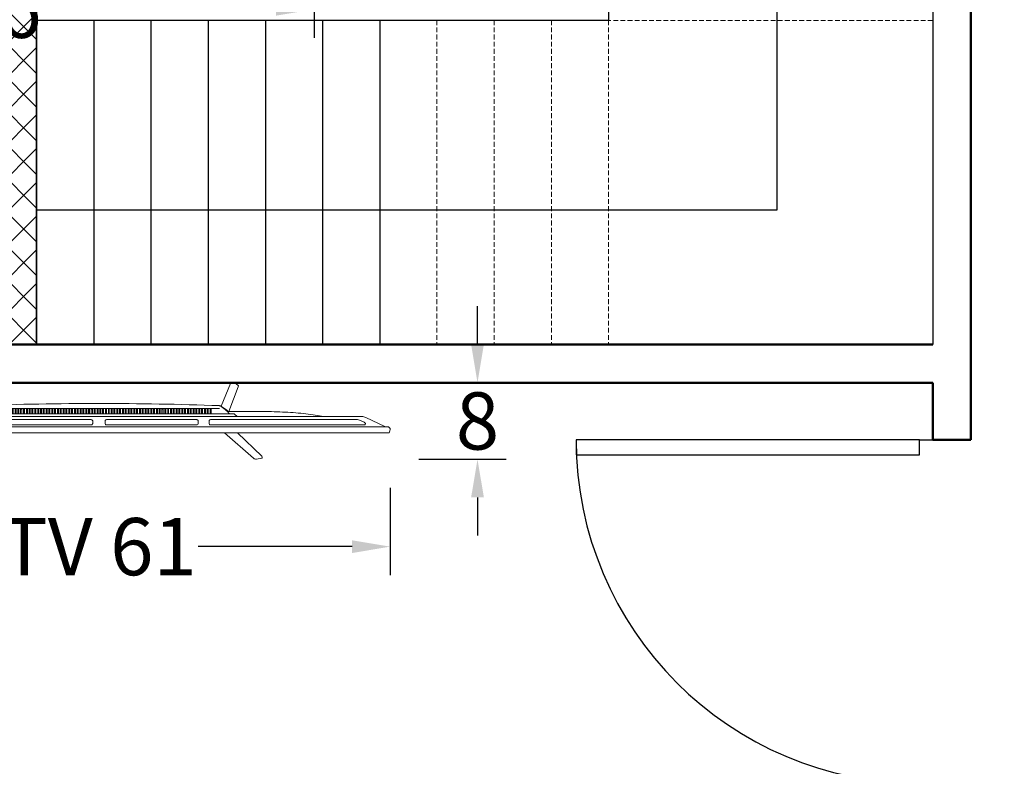
# Model space of a CAD drawing. Units: inches. Extents: x -466983 to 1020, y 324 to 318697.
# Tile 29 of 97: x 714 to 817, y 658 to 736. Entities that reach past the tile are written whole.
import ezdxf

# ---------------------------------------------------------------- set-up
doc = ezdxf.new("R2010")
doc.units = ezdxf.units.IN
doc.header["$MEASUREMENT"] = 0
doc.linetypes.add('DASHED', pattern=[0.75, 0.5, -0.25])
for name, color, linetype, lineweight in [('A-ANNO-DIMS', 2, 'Continuous', 18), ('A-DOOR', 3, 'Continuous', 25), ('A-FLOR-PATT', 252, 'Continuous', 13), ('A-FLOR-STRS', 30, 'Continuous', 25), ('A-FLOR-STRS-OVHD', 30, 'DASHED', 18), ('A-FURN', 8, 'Continuous', 18), ('A-WALL', 7, 'Continuous', 50)]:
    doc.layers.add(name, color=color, linetype=linetype, lineweight=lineweight)
doc.styles.get("Standard").update_dxf_attribs({"font": 'arial.ttf'})
doc.dimstyles.get("Standard").update_dxf_attribs({"dimtxt": 6, "dimasz": 4, "dimexe": 3, "dimexo": 3, "dimgap": 0.09, "dimtad": 0, "dimtih": 1, "dimtoh": 1, "dimdec": 1, "dimzin": 0, "dimdsep": 46, "dimlunit": 3, "dimtxsty": 'Standard', "dimcen": 0.09, "dimadec": 0, "dimazin": 0, "dimtfac": 1, "dimtdec": 1, "dimtofl": 0, "dimtmove": 0, "dimatfit": 3, "dimfxl": 1, "dimtolj": 1, "dimtzin": 0, "dimarcsym": 0})

# ---------------------------------------------------------------- blocks, each defined once
blk = doc.blocks.new('B2')
at = {"color": 0}
for points in [[(-161.1, -3.4), (-173.3, 26.2, 0.359324), (-175.3, 27.3, 0.097501), (-182.8, 24.2, 0.350578), (-183.5, 22.1), (-171.1, -10.4)], [(161.1, -3.4), (173.3, 26.2, -0.359324), (175.3, 27.3, -0.097501), (182.8, 24.2, -0.350578), (183.5, 22.1), (171.1, -10.4)], [(-295.5, -17), (-282, -15, -0.02037), (-255.8, -12, -0.012056), (-227.2, -10.7), (-169.3, -10.7)], [(-172.1, -13.6, -0.072098), (-159.2, -3, -0.121861), (-158.4, -2.8)], [(-170.1, -10.6, -0.053076), (-160.2, -2.9), (-158.4, -2.8)], [(-147.6, -13.6), (-147.6, -7.5, -0.414214), (-147.4, -7.3), (-146.5, -7.3, -0.414214), (-146.3, -7.5), (-146.3, -13.6)], [(-143.9, -13.6), (-143.9, -7.5, -0.414214), (-143.7, -7.3), (-142.7, -7.3, -0.414214), (-142.6, -7.5), (-142.6, -13.6)], [(-140.2, -13.6), (-140.2, -7.5, -0.414214), (-140, -7.3), (-139, -7.3, -0.414214), (-138.8, -7.5), (-138.8, -13.6)], [(-136.4, -13.6), (-136.4, -7.5, -0.414214), (-136.3, -7.3), (-135.3, -7.3, -0.414214), (-135.1, -7.5), (-135.1, -13.6)], [(-132.7, -13.6), (-132.7, -7.5, -0.414214), (-132.5, -7.3), (-131.6, -7.3, -0.414214), (-131.4, -7.5), (-131.4, -13.6)], [(-129, -13.6), (-129, -7.5, -0.414214), (-128.8, -7.3), (-127.9, -7.3, -0.414214), (-127.7, -7.5), (-127.7, -13.6)], [(-125.3, -13.6), (-125.3, -7.5, -0.414214), (-125.1, -7.3), (-124.1, -7.3, -0.414214), (-124, -7.5), (-124, -13.6)], [(-121.6, -13.6), (-121.6, -7.5, -0.414214), (-121.4, -7.3), (-120.4, -7.3, -0.414214), (-120.2, -7.5), (-120.2, -13.6)], [(-117.8, -13.6), (-117.8, -7.5, -0.414214), (-117.7, -7.3), (-116.7, -7.3, -0.414214), (-116.5, -7.5), (-116.5, -13.6)], [(-114.1, -13.6), (-114.1, -7.5, -0.414214), (-113.9, -7.3), (-113, -7.3, -0.414214), (-112.8, -7.5), (-112.8, -13.6)], [(-110.4, -13.6), (-110.4, -7.5, -0.414214), (-110.2, -7.3), (-109.3, -7.3, -0.414214), (-109.1, -7.5), (-109.1, -13.6)], [(-106.7, -13.6), (-106.7, -7.5, -0.414214), (-106.5, -7.3), (-105.5, -7.3, -0.414214), (-105.4, -7.5), (-105.4, -13.6)], [(-103, -13.6), (-103, -7.5, -0.414214), (-102.8, -7.3), (-101.8, -7.3, -0.414214), (-101.6, -7.5), (-101.6, -13.6)], [(-99.2, -13.6), (-99.2, -7.5, -0.414214), (-99.1, -7.3), (-98.1, -7.3, -0.414214), (-97.9, -7.5), (-97.9, -13.6)], [(-95.5, -13.6), (-95.5, -7.5, -0.414214), (-95.3, -7.3), (-94.4, -7.3, -0.414214), (-94.2, -7.5), (-94.2, -13.6)], [(-91.8, -13.6), (-91.8, -7.5, -0.414214), (-91.6, -7.3), (-90.7, -7.3, -0.414214), (-90.5, -7.5), (-90.5, -13.6)], [(-88.1, -13.6), (-88.1, -7.5, -0.414214), (-87.9, -7.3), (-86.9, -7.3, -0.414214), (-86.8, -7.5), (-86.8, -13.6)], [(-84.4, -13.6), (-84.4, -7.5, -0.414214), (-84.2, -7.3), (-83.2, -7.3, -0.414214), (-83, -7.5), (-83, -13.6)], [(-80.6, -13.6), (-80.6, -7.5, -0.414214), (-80.5, -7.3), (-79.5, -7.3, -0.414214), (-79.3, -7.5), (-79.3, -13.6)], [(-76.9, -13.6), (-76.9, -7.5, -0.414214), (-76.7, -7.3), (-75.8, -7.3, -0.414214), (-75.6, -7.5), (-75.6, -13.6)], [(-73.2, -13.6), (-73.2, -7.5, -0.414214), (-73, -7.3), (-72.1, -7.3, -0.414214), (-71.9, -7.5), (-71.9, -13.6)], [(-69.5, -13.6), (-69.5, -7.5, -0.414214), (-69.3, -7.3), (-68.3, -7.3, -0.414214), (-68.2, -7.5), (-68.2, -13.6)], [(-65.8, -13.6), (-65.8, -7.5, -0.414214), (-65.6, -7.3), (-64.6, -7.3, -0.414214), (-64.4, -7.5), (-64.4, -13.6)], [(-62, -13.6), (-62, -7.5, -0.414214), (-61.9, -7.3), (-60.9, -7.3, -0.414214), (-60.7, -7.5), (-60.7, -13.6)], [(-58.3, -13.6), (-58.3, -7.5, -0.414214), (-58.1, -7.3), (-57.2, -7.3, -0.414214), (-57, -7.5), (-57, -13.6)], [(-54.6, -13.6), (-54.6, -7.5, -0.414214), (-54.4, -7.3), (-53.5, -7.3, -0.414214), (-53.3, -7.5), (-53.3, -13.6)], [(-50.9, -13.6), (-50.9, -7.5, -0.414214), (-50.7, -7.3), (-49.7, -7.3, -0.414214), (-49.6, -7.5), (-49.6, -13.6)], [(-47.2, -13.6), (-47.2, -7.5, -0.414214), (-47, -7.3), (-46, -7.3, -0.414214), (-45.8, -7.5), (-45.8, -13.6)], [(-43.4, -13.6), (-43.4, -7.5, -0.414214), (-43.3, -7.3), (-42.3, -7.3, -0.414214), (-42.1, -7.5), (-42.1, -13.6)], [(-39.7, -13.6), (-39.7, -7.5, -0.414214), (-39.5, -7.3), (-38.6, -7.3, -0.414214), (-38.4, -7.5), (-38.4, -13.6)], [(-36, -13.6), (-36, -7.5, -0.414214), (-35.8, -7.3), (-34.9, -7.3, -0.414214), (-34.7, -7.5), (-34.7, -13.6)], [(-32.3, -13.6), (-32.3, -7.5, -0.414214), (-32.1, -7.3), (-31.1, -7.3, -0.414214), (-31, -7.5), (-31, -13.6)], [(-28.6, -13.6), (-28.6, -7.5, -0.414214), (-28.4, -7.3), (-27.4, -7.3, -0.414214), (-27.2, -7.5), (-27.2, -13.6)], [(-24.8, -13.6), (-24.8, -7.5, -0.414214), (-24.7, -7.3), (-23.7, -7.3, -0.414214), (-23.5, -7.5), (-23.5, -13.6)], [(-21.1, -13.6), (-21.1, -7.5, -0.414214), (-20.9, -7.3), (-20, -7.3, -0.414214), (-19.8, -7.5), (-19.8, -13.6)], [(-17.4, -13.6), (-17.4, -7.5, -0.414214), (-17.2, -7.3), (-16.3, -7.3, -0.414214), (-16.1, -7.5), (-16.1, -13.6)], [(-13.7, -13.6), (-13.7, -7.5, -0.414214), (-13.5, -7.3), (-12.5, -7.3, -0.414214), (-12.4, -7.5), (-12.4, -13.6)], [(-10, -13.6), (-10, -7.5, -0.414214), (-9.8, -7.3), (-8.8, -7.3, -0.414214), (-8.6, -7.5), (-8.6, -13.6)], [(-6.2, -13.6), (-6.2, -7.5, -0.414214), (-6.1, -7.3), (-5.1, -7.3, -0.414214), (-4.9, -7.5), (-4.9, -13.6)], [(-2.5, -13.6), (-2.5, -7.5, -0.414214), (-2.3, -7.3), (-1.4, -7.3, -0.414214), (-1.2, -7.5), (-1.2, -13.6)], [(2.5, -13.6), (2.5, -7.5, 0.414214), (2.3, -7.3), (1.4, -7.3, 0.414214), (1.2, -7.5), (1.2, -13.6)], [(6.2, -13.6), (6.2, -7.5, 0.414214), (6.1, -7.3), (5.1, -7.3, 0.414214), (4.9, -7.5), (4.9, -13.6)], [(10, -13.6), (10, -7.5, 0.414214), (9.8, -7.3), (8.8, -7.3, 0.414214), (8.6, -7.5), (8.6, -13.6)], [(13.7, -13.6), (13.7, -7.5, 0.414214), (13.5, -7.3), (12.5, -7.3, 0.414214), (12.4, -7.5), (12.4, -13.6)], [(17.4, -13.6), (17.4, -7.5, 0.414214), (17.2, -7.3), (16.3, -7.3, 0.414214), (16.1, -7.5), (16.1, -13.6)], [(21.1, -13.6), (21.1, -7.5, 0.414214), (20.9, -7.3), (20, -7.3, 0.414214), (19.8, -7.5), (19.8, -13.6)], [(24.8, -13.6), (24.8, -7.5, 0.414214), (24.7, -7.3), (23.7, -7.3, 0.414214), (23.5, -7.5), (23.5, -13.6)], [(28.6, -13.6), (28.6, -7.5, 0.414214), (28.4, -7.3), (27.4, -7.3, 0.414214), (27.2, -7.5), (27.2, -13.6)], [(32.3, -13.6), (32.3, -7.5, 0.414214), (32.1, -7.3), (31.1, -7.3, 0.414214), (31, -7.5), (31, -13.6)], [(36, -13.6), (36, -7.5, 0.414214), (35.8, -7.3), (34.9, -7.3, 0.414214), (34.7, -7.5), (34.7, -13.6)], [(39.7, -13.6), (39.7, -7.5, 0.414214), (39.5, -7.3), (38.6, -7.3, 0.414214), (38.4, -7.5), (38.4, -13.6)], [(43.4, -13.6), (43.4, -7.5, 0.414214), (43.3, -7.3), (42.3, -7.3, 0.414214), (42.1, -7.5), (42.1, -13.6)], [(47.2, -13.6), (47.2, -7.5, 0.414214), (47, -7.3), (46, -7.3, 0.414214), (45.8, -7.5), (45.8, -13.6)], [(50.9, -13.6), (50.9, -7.5, 0.414214), (50.7, -7.3), (49.7, -7.3, 0.414214), (49.6, -7.5), (49.6, -13.6)], [(54.6, -13.6), (54.6, -7.5, 0.414214), (54.4, -7.3), (53.5, -7.3, 0.414214), (53.3, -7.5), (53.3, -13.6)], [(58.3, -13.6), (58.3, -7.5, 0.414214), (58.1, -7.3), (57.2, -7.3, 0.414214), (57, -7.5), (57, -13.6)], [(62, -13.6), (62, -7.5, 0.414214), (61.9, -7.3), (60.9, -7.3, 0.414214), (60.7, -7.5), (60.7, -13.6)], [(65.8, -13.6), (65.8, -7.5, 0.414214), (65.6, -7.3), (64.6, -7.3, 0.414214), (64.4, -7.5), (64.4, -13.6)], [(69.5, -13.6), (69.5, -7.5, 0.414214), (69.3, -7.3), (68.3, -7.3, 0.414214), (68.2, -7.5), (68.2, -13.6)], [(73.2, -13.6), (73.2, -7.5, 0.414214), (73, -7.3), (72.1, -7.3, 0.414214), (71.9, -7.5), (71.9, -13.6)], [(76.9, -13.6), (76.9, -7.5, 0.414214), (76.7, -7.3), (75.8, -7.3, 0.414214), (75.6, -7.5), (75.6, -13.6)], [(80.6, -13.6), (80.6, -7.5, 0.414214), (80.5, -7.3), (79.5, -7.3, 0.414214), (79.3, -7.5), (79.3, -13.6)], [(84.4, -13.6), (84.4, -7.5, 0.414214), (84.2, -7.3), (83.2, -7.3, 0.414214), (83, -7.5), (83, -13.6)], [(88.1, -13.6), (88.1, -7.5, 0.414214), (87.9, -7.3), (86.9, -7.3, 0.414214), (86.8, -7.5), (86.8, -13.6)], [(91.8, -13.6), (91.8, -7.5, 0.414214), (91.6, -7.3), (90.7, -7.3, 0.414214), (90.5, -7.5), (90.5, -13.6)], [(95.5, -13.6), (95.5, -7.5, 0.414214), (95.3, -7.3), (94.4, -7.3, 0.414214), (94.2, -7.5), (94.2, -13.6)], [(99.2, -13.6), (99.2, -7.5, 0.414214), (99.1, -7.3), (98.1, -7.3, 0.414214), (97.9, -7.5), (97.9, -13.6)], [(103, -13.6), (103, -7.5, 0.414214), (102.8, -7.3), (101.8, -7.3, 0.414214), (101.6, -7.5), (101.6, -13.6)], [(106.7, -13.6), (106.7, -7.5, 0.414214), (106.5, -7.3), (105.5, -7.3, 0.414214), (105.4, -7.5), (105.4, -13.6)], [(110.4, -13.6), (110.4, -7.5, 0.414214), (110.2, -7.3), (109.3, -7.3, 0.414214), (109.1, -7.5), (109.1, -13.6)], [(114.1, -13.6), (114.1, -7.5, 0.414214), (113.9, -7.3), (113, -7.3, 0.414214), (112.8, -7.5), (112.8, -13.6)], [(117.8, -13.6), (117.8, -7.5, 0.414214), (117.7, -7.3), (116.7, -7.3, 0.414214), (116.5, -7.5), (116.5, -13.6)], [(121.6, -13.6), (121.6, -7.5, 0.414214), (121.4, -7.3), (120.4, -7.3, 0.414214), (120.2, -7.5), (120.2, -13.6)], [(125.3, -13.6), (125.3, -7.5, 0.414214), (125.1, -7.3), (124.1, -7.3, 0.414214), (124, -7.5), (124, -13.6)], [(129, -13.6), (129, -7.5, 0.414214), (128.8, -7.3), (127.9, -7.3, 0.414214), (127.7, -7.5), (127.7, -13.6)], [(132.7, -13.6), (132.7, -7.5, 0.414214), (132.5, -7.3), (131.6, -7.3, 0.414214), (131.4, -7.5), (131.4, -13.6)], [(136.4, -13.6), (136.4, -7.5, 0.414214), (136.3, -7.3), (135.3, -7.3, 0.414214), (135.1, -7.5), (135.1, -13.6)], [(140.2, -13.6), (140.2, -7.5, 0.414214), (140, -7.3), (139, -7.3, 0.414214), (138.8, -7.5), (138.8, -13.6)], [(143.9, -13.6), (143.9, -7.5, 0.414214), (143.7, -7.3), (142.7, -7.3, 0.414214), (142.6, -7.5), (142.6, -13.6)], [(147.6, -13.6), (147.6, -7.5, 0.414214), (147.4, -7.3), (146.5, -7.3, 0.414214), (146.3, -7.5), (146.3, -13.6)], [(172.1, -13.6, 0.072098), (159.2, -3, 0.121861), (158.4, -2.8)], [(170.1, -10.6, 0.053076), (160.2, -2.9), (158.4, -2.8)], [(295.5, -17), (282, -15, 0.02037), (255.8, -12, 0.012056), (227.2, -10.7), (169.3, -10.7)], [(-381.9, -38.8, -0.13121), (-383.2, -32.7, -0.169032), (-383, -32.3), (-381.8, -31.1, -0.205713), (-381.3, -30.9), (-378.5, -30.9, 0.118206), (-376.2, -30.4), (-351.4, -18.4, -0.105648), (-345.8, -17), (0, -17)], [(-339.3, -21.2), (-339.3, -21.2, 0.099639), (-344.3, -22.2), (-349.2, -24.6, 0.215889), (-350.7, -26.3, 0.476075), (-349.4, -28, 0.244765)], [(-181.8, -17), (-178.5, -14, -0.213415), (-177.3, -13.6), (0, -13.6)], [(-146.8, -28, 0.414214), (-145, -26.2), (-145, -23, 0.414214), (-146.8, -21.2)], [(-128.8, -28, -0.414214), (-130.6, -26.2), (-130.6, -23, -0.414214), (-128.8, -21.2)], [(-10, -28, 0.414214), (-8.2, -26.2), (-8.2, -23, 0.414214), (-10, -21.2)], [(181.8, -17), (178.5, -14, 0.213415), (177.3, -13.6), (0, -13.6)], [(381.9, -38.8, 0.13121), (383.2, -32.7, 0.169032), (383, -32.3), (381.8, -31.1, 0.205713), (381.3, -30.9), (378.5, -30.9, -0.118206), (376.2, -30.4), (351.4, -18.4, 0.105648), (345.8, -17), (0, -17)], [(10, -28, -0.414214), (8.2, -26.2), (8.2, -23, -0.414214), (10, -21.2)], [(128.8, -28, 0.414214), (130.6, -26.2), (130.6, -23, 0.414214), (128.8, -21.2)], [(146.8, -28, -0.414214), (145, -26.2), (145, -23, -0.414214), (146.8, -21.2)], [(339.3, -21.2), (339.3, -21.2, -0.099639), (344.3, -22.2), (349.2, -24.6, -0.215889), (350.7, -26.3, -0.476075), (349.4, -28, -0.244765)], [(-182.5, -38.8), (-214.4, -69.1, 0.250582), (-215, -71, 0.266718), (-214.3, -71.9, 0.084688)], [(-214.3, -71.9), (-207.3, -73.1, 0.211205), (-203.3, -72.1), (-165.2, -38.8)], [(214.3, -71.9), (207.3, -73.1, -0.211205), (203.3, -72.1), (165.2, -38.8)], [(182.5, -38.8), (214.4, -69.1, -0.250582), (215, -71, -0.266718), (214.3, -71.9, -0.084688)]]:
    blk.add_lwpolyline(points, format="xyb", dxfattribs=at)
for points in [[(-158.6, -6.5), (0, -6.5)], [(158.6, -6.5), (0, -6.5)], [(-339.3, -21.2), (-146.8, -21.2)], [(-128.8, -21.2), (-10, -21.2)], [(128.8, -21.2), (10, -21.2)], [(339.3, -21.2), (146.8, -21.2)], [(-381.9, -38.8), (0, -38.8)], [(-378.5, -30.9), (0, -30.9)], [(-349.4, -28), (-146.8, -28)], [(-128.8, -28), (-10, -28)], [(378.5, -30.9), (0, -30.9)], [(381.9, -38.8), (0, -38.8)], [(128.8, -28), (10, -28)], [(349.4, -28), (146.8, -28)]]:
    blk.add_lwpolyline(points, dxfattribs=at)
for centre, radius, start, end in [((0, -4564), 4564, 90, 91.9893), ((0, -4564), 4564, 88.0107, 90), ((-170.5, -10.1), 0.6, 200.9784, 314.0295), ((170.5, -10.1), 0.6, 225.9705, 339.0216)]:
    blk.add_arc(centre, radius, start, end, dxfattribs=at)
blk = doc.blocks.new('*U39')
for p, q in [((0, 0), (0, -6)), ((-40, 0), (-40, -6))]:
    blk.add_line(p, q)
blk.add_lwpolyline([(0, 0), (0, 40), (-1.75, 40), (-1.75, 0)], close=True)
blk.add_arc((0, 0), 40, 90, 180)
blk = doc.blocks.new('*D101')
at = {"layer": 'A-ANNO-DIMS', "color": 0, "lineweight": -2, "transparency": 16777216}
for p, q in [((691.81, 686.91), (691.81, 677.75)), ((752.9, 686.91), (752.9, 677.75)), ((695.81, 680.75), (711.95, 680.75)), ((748.9, 680.75), (732.76, 680.75))]:
    blk.add_line(p, q, dxfattribs=at)
at = {"layer": 'A-ANNO-DIMS', "color": 0, "transparency": 16777216}
for points in [[(695.81, 681.42), (695.81, 680.08), (691.81, 680.75)], [(748.9, 681.42), (748.9, 680.08), (752.9, 680.75)]]:
    blk.add_solid(points, dxfattribs=at)
at = {"layer": 'Defpoints', "color": 0, "transparency": 16777216}
for p in [(691.81, 689.91), (752.9, 689.91), (752.9, 680.75)]:
    blk.add_point(p, dxfattribs=at)
at = {"layer": 'A-ANNO-DIMS', "color": 0, "transparency": 16777216, "insert": (722.35, 680.75), "char_height": 6, "attachment_point": 5}
blk.add_mtext('\\A1;TV 61', dxfattribs=at)
blk = doc.blocks.new('*D102')
at = {"layer": 'A-ANNO-DIMS', "color": 0, "lineweight": -2, "transparency": 16777216}
for p, q in [((762.06, 701.95), (762.06, 705.95)), ((755.9, 697.95), (765.06, 697.95)), ((755.9, 689.91), (765.06, 689.91)), ((762.06, 685.91), (762.06, 681.91))]:
    blk.add_line(p, q, dxfattribs=at)
at = {"layer": 'A-ANNO-DIMS', "color": 0, "transparency": 16777216}
for points in [[(761.39, 701.95), (762.73, 701.95), (762.06, 697.95)], [(761.39, 685.91), (762.73, 685.91), (762.06, 689.91)]]:
    blk.add_solid(points, dxfattribs=at)
at = {"layer": 'Defpoints', "color": 0, "transparency": 16777216}
for p in [(752.9, 697.95), (762.06, 697.95), (752.9, 689.91)]:
    blk.add_point(p, dxfattribs=at)
at = {"layer": 'A-ANNO-DIMS', "color": 0, "transparency": 16777216, "insert": (762.06, 693.93), "char_height": 6, "attachment_point": 5}
blk.add_mtext('\\A1;8', dxfattribs=at)
blk = doc.blocks.new('*D112')
at = {"layer": 'A-ANNO-DIMS', "color": 0, "lineweight": -2, "transparency": 16777216}
for p, q in [((678.65, 751.43), (678.65, 734.1)), ((744.94, 751.43), (744.94, 734.1)), ((682.65, 737.1), (707.39, 737.1)), ((740.94, 737.1), (716.2, 737.1))]:
    blk.add_line(p, q, dxfattribs=at)
at = {"layer": 'A-ANNO-DIMS', "color": 0, "transparency": 16777216}
for points in [[(682.65, 737.76), (682.65, 736.43), (678.65, 737.1)], [(740.94, 737.76), (740.94, 736.43), (744.94, 737.1)]]:
    blk.add_solid(points, dxfattribs=at)
at = {"layer": 'Defpoints', "color": 0, "transparency": 16777216}
for p in [(678.65, 754.43), (744.94, 754.43), (744.94, 737.1)]:
    blk.add_point(p, dxfattribs=at)
at = {"layer": 'A-ANNO-DIMS', "color": 0, "transparency": 16777216, "insert": (711.79, 737.1), "char_height": 6, "attachment_point": 5}
blk.add_mtext('\\A1;66', dxfattribs=at)

msp = doc.modelspace()

# ---------------------------------------------------------------- hatches: boundary and pattern name
at = {"layer": 'A-FLOR-PATT', "transparency": 33554572}
h = msp.add_hatch(dxfattribs=at)
h.set_pattern_fill('ANSI37', color=256, scale=30)
h.set_pattern_definition([(45, (-1212.4137, -290.035), (-2.6516504, 2.6516504), []), (135, (-1212.4137, -290.035), (-2.6516504, -2.6516504), [])])
h.paths.add_polyline_path([(901.81, 1075.94), (900.61, 1075.94), (900.61, 1065.39), (899.39, 1065.39), (898.09, 1065.39), (892.84, 1058.71, -0.258377), (892.19, 1058.35), (879.98, 1058.35, -0.20177), (879.44, 1058.58), (874.08, 1065.39), (872.78, 1065.39), (871.56, 1065.39), (871.56, 1075.94), (813.81, 1075.94), (813.81, 1044.79), (832.39, 1044.79, -0.394795), (848.66, 1028.54), (848.66, 1009.94), (901.81, 1009.94), (901.81, 1015.94), (901.31, 1015.94), (871.31, 1015.94), (871.31, 1017.25), (871.33, 1017.25, -0.401453), (901.31, 1045.94), (901.81, 1045.94)])
edge = h.paths.add_edge_path(flags=16)
edge.add_line((847.77, 1068.95), (847.77, 1073.71))
edge.add_arc((849.23, 1073.71), 1.45, 90, 180, ccw=False)
edge.add_line((849.23, 1075.16), (864.49, 1075.16))
edge.add_arc((864.49, 1073.71), 1.45, 0, 90, ccw=False)
edge.add_line((865.95, 1073.71), (865.95, 1069))
edge.add_arc((832.64, 1068.98), 33.3, -20.6123, 0.0472, ccw=False)
edge.add_ellipse((856.86, 1058.48), major_axis=(0, 10.21), ratio=0.685919, start_angle=100.0088, end_angle=259.9912, ccw=False)
edge.add_arc((881.07, 1068.98), 33.3, 180.0472, 200.6123, ccw=False)
h.paths.add_polyline_path([(853.15, 1066.48), (853.15, 1066.45), (853.15, 1066.45, 0.433107), (852.92, 1066.68), (852.92, 1066.45), (853.15, 1066.45), (853.15, 1066.48), (853.09, 1066.61, 0.697939), (852.7, 1066.45), (852.7, 1066.45), (852.7, 1066.48), (852.92, 1067), (852.92, 1066.68, -0.396254)], flags=0)
h.paths.add_polyline_path([(861.02, 1066.48), (861.02, 1066.45), (861.02, 1066.45, 0.416404), (860.8, 1066.68), (860.8, 1066.45), (861.02, 1066.45), (861.02, 1066.48), (860.97, 1066.61, 0.713344), (860.57, 1066.45), (860.57, 1066.45), (860.57, 1066.48), (860.8, 1067), (860.8, 1066.68, -0.379973)], flags=0)
edge = h.paths.add_edge_path(flags=0)
edge.add_spline(control_points=[(861.13, 1065.79), (861.47, 1065.25), (861.61, 1065.02), (861.98, 1064.37), (862.19, 1063.94), (862.56, 1063.04), (862.72, 1062.56), (862.99, 1061.58), (863.09, 1061.07), (863.25, 1060.03), (863.29, 1059.5), (863.33, 1058.44), (863.32, 1057.91), (863.24, 1056.85), (863.17, 1056.33), (862.97, 1055.31), (862.84, 1054.81), (862.54, 1053.85), (862.36, 1053.39), (861.95, 1052.52), (861.73, 1052.12), (861.23, 1051.36), (860.97, 1051.02), (860.4, 1050.39), (860.11, 1050.12), (859.49, 1049.65), (859.18, 1049.45), (858.53, 1049.13), (858.2, 1049.01), (857.53, 1048.85), (857.2, 1048.81), (856.52, 1048.81), (856.19, 1048.85), (855.52, 1049.01), (855.19, 1049.13), (854.54, 1049.45), (854.23, 1049.64), (853.61, 1050.12), (853.32, 1050.39), (852.75, 1051.01), (852.49, 1051.36), (852, 1052.11), (851.77, 1052.52), (851.36, 1053.39), (851.18, 1053.85), (850.88, 1054.81), (850.75, 1055.31), (850.55, 1056.33), (850.48, 1056.85), (850.4, 1057.9), (850.39, 1058.44), (850.43, 1059.5), (850.47, 1060.03), (850.63, 1061.07), (850.73, 1061.58), (851, 1062.56), (851.16, 1063.04), (851.53, 1063.94), (851.73, 1064.37), (852.11, 1065.02), (852.25, 1065.25), (852.61, 1065.73)], knot_values=[3.915332, 3.915332, 3.915332, 3.915332, 4.013468, 4.013468, 4.175532, 4.175532, 4.337596, 4.337596, 4.49966, 4.49966, 4.661724, 4.661724, 4.823788, 4.823788, 4.985852, 4.985852, 5.147916, 5.147916, 5.30998, 5.30998, 5.472044, 5.472044, 5.634109, 5.634109, 5.796173, 5.796173, 5.958237, 5.958237, 6.120301, 6.120301, 6.282365, 6.282365, 6.444429, 6.444429, 6.606493, 6.606493, 6.768557, 6.768557, 6.930621, 6.930621, 7.092685, 7.092685, 7.254749, 7.254749, 7.416813, 7.416813, 7.578878, 7.578878, 7.740942, 7.740942, 7.903006, 7.903006, 8.06507, 8.06507, 8.227134, 8.227134, 8.389198, 8.389198, 8.551262, 8.551262, 8.65037, 8.65037, 8.65037, 8.65037], degree=3, periodic=0)
edge.add_line((852.64, 1065.79), (861.13, 1065.79))
edge = h.paths.add_edge_path(flags=0)
edge.add_ellipse((856.85, 1057.74), major_axis=(0, 7.79), ratio=0.687861, start_angle=0, end_angle=360)
h.paths.add_polyline_path([(848.86, 1069.39), (848.86, 1073.96, -0.414214), (849.95, 1075.05), (863.77, 1075.05, -0.414214), (864.86, 1073.96), (864.86, 1069.39, -0.388936), (864.52, 1069.03, -0.043561), (849.2, 1069.03, -0.388936)], flags=0)
h.paths.add_polyline_path([(853.1, 1068.11, -1), (852.68, 1068.11, -1)], flags=0)
edge = h.paths.add_edge_path(flags=0)
edge.add_ellipse((856.86, 1057.34), major_axis=(0, 2.21), ratio=0.657164, start_angle=0, end_angle=360)
h.paths.add_polyline_path([(861.04, 1068.11, -1), (860.62, 1068.11, -1)], flags=0)
edge = h.paths.add_edge_path()
edge.add_line((573.95, 1057.34), (573.95, 1075.94))
edge.add_line((573.95, 1075.94), (558.73, 1075.94))
edge.add_line((558.73, 1075.94), (558.73, 1065.39))
edge.add_line((558.73, 1065.39), (557.51, 1065.39))
edge.add_line((557.51, 1065.39), (556.21, 1065.39))
edge.add_line((556.21, 1065.39), (550.95, 1058.71))
edge.add_arc((550.3, 1059.12), 0.765, 270, 327.9483, ccw=False)
edge.add_line((550.3, 1058.35), (538.1, 1058.35))
edge.add_arc((538.1, 1059.12), 0.765, 224.3704, 270, ccw=False)
edge.add_line((537.55, 1058.58), (532.2, 1065.39))
edge.add_line((532.2, 1065.39), (530.9, 1065.39))
edge.add_line((530.9, 1065.39), (529.67, 1065.39))
edge.add_line((529.67, 1065.39), (529.67, 1075.94))
edge.add_line((529.67, 1075.94), (520.81, 1075.94))
edge.add_line((520.81, 1075.94), (520.81, 1045.94))
edge.add_line((520.81, 1045.94), (521.31, 1045.94))
edge.add_arc((521.31, 1015.94), 30, 2.5075, 90, ccw=False)
edge.add_line((551.28, 1017.25), (551.31, 1017.25))
edge.add_line((551.31, 1017.25), (551.31, 1015.94))
edge.add_line((551.31, 1015.94), (520.81, 1015.94))
edge.add_line((520.81, 1015.94), (520.81, 1009.94))
edge.add_line((520.81, 1009.94), (559.19, 1010.4))
edge.add_arc((559.19, 1011.86), 1.45, 180, 270, ccw=False)
edge.add_line((557.74, 1011.86), (557.74, 1016.56))
edge.add_arc((591.04, 1016.59), 33.3, 159.3877, 180.0472, ccw=False)
edge.add_ellipse((566.82, 1027.08), major_axis=(0, 10.21), ratio=0.685919, start_angle=280.0088, end_angle=439.9912, ccw=False)
edge.add_arc((542.61, 1016.59), 33.3, 0.0472, 20.6123, ccw=False)
edge.add_line((575.91, 1016.62), (575.91, 1011.86))
edge.add_arc((574.46, 1011.86), 1.45, -90, 0, ccw=False)
edge.add_line((574.46, 1010.4), (608.81, 1009.94))
edge.add_line((608.81, 1009.94), (608.81, 1041.09))
edge.add_line((608.81, 1041.09), (590.22, 1041.09))
edge.add_arc((590.78, 1057.91), 16.83, 181.9277, 268.1032, ccw=False)
edge = h.paths.add_edge_path()
edge.add_ellipse((494.24, 583.62), major_axis=(0, 10.21), ratio=0.685919, start_angle=280.0088, end_angle=439.9912, ccw=False)
edge.add_arc((470.03, 573.12), 33.3, 0.0472, 20.6123, ccw=False)
edge.add_line((503.33, 573.15), (503.33, 568.39))
edge.add_arc((501.88, 568.39), 1.45, -90, 0, ccw=False)
edge.add_line((501.88, 566.94), (539.81, 566.94))
edge.add_line((539.81, 566.94), (539.81, 572.94))
edge.add_line((539.81, 572.94), (539.31, 572.94))
edge.add_line((539.31, 572.94), (509.31, 572.94))
edge.add_line((509.31, 572.94), (509.31, 574.25))
edge.add_line((509.31, 574.25), (509.33, 574.25))
edge.add_arc((539.31, 572.94), 30, 90, 177.4925, ccw=False)
edge.add_line((539.31, 602.94), (539.81, 602.94))
edge.add_line((539.81, 602.94), (539.81, 626.94))
edge.add_line((539.81, 626.94), (531.77, 626.94))
edge.add_line((531.77, 626.94), (531.77, 616.39))
edge.add_line((531.77, 616.39), (530.55, 616.39))
edge.add_line((530.55, 616.39), (529.25, 616.39))
edge.add_line((529.25, 616.39), (523.71, 609.35))
edge.add_line((523.71, 609.35), (510.78, 609.35))
edge.add_line((510.78, 609.35), (505.24, 616.39))
edge.add_line((505.24, 616.39), (503.94, 616.39))
edge.add_line((503.94, 616.39), (502.72, 616.39))
edge.add_line((502.72, 616.39), (502.72, 626.94))
edge.add_line((502.72, 626.94), (481.7, 626.94))
edge.add_line((481.7, 626.94), (481.7, 611))
edge.add_arc((467.27, 611.47), 14.44, 271.9277, 358.1032, ccw=False)
edge.add_line((467.76, 597.05), (451.81, 597.05))
edge.add_line((451.81, 597.05), (451.81, 584.4))
edge.add_line((451.81, 584.4), (451.81, 566.94))
edge.add_line((451.81, 566.94), (486.61, 566.94))
edge.add_arc((486.61, 568.39), 1.45, 180, 270, ccw=False)
edge.add_line((485.16, 568.39), (485.16, 573.1))
edge.add_arc((518.46, 573.12), 33.3, 159.3877, 180.0472, ccw=False)
h.paths.add_polyline_path([(836.26, 1020.73), (879.89, 1020.73), (879.89, 1039.39), (836.26, 1039.39)], flags=25)
h.paths.add_polyline_path([(549.99, 1036.75), (593.61, 1036.75), (593.61, 1055.41), (549.99, 1055.41)], flags=24)
h.paths.add_polyline_path([(475.12, 595.6), (518.75, 595.6), (518.75, 614.25), (475.12, 614.25)], flags=24)
h = msp.add_hatch(dxfattribs=at)
h.set_pattern_fill('ANSI37', color=256, scale=20)
h.set_pattern_definition([(45, (-1212.4137, -290.035), (-1.767767, 1.767767), []), (135, (-1212.4137, -290.035), (-1.767767, -1.767767), [])])
h.paths.add_polyline_path([(809.81, 870.94), (809.81, 888.15), (807, 888.15), (802.66, 888.15), (789.38, 888.15), (786.28, 888.15, -0.414214), (785.5, 888.94), (785.5, 900.2), (785.5, 908.47, -0.414214), (786.81, 909.78, -0.414214), (785.5, 911.09), (785.5, 929.1, -0.414214), (786.81, 930.41, -0.414214), (785.5, 931.72), (785.5, 931.9, -0.414214), (784.19, 930.59), (766.72, 930.59, -0.412359), (765.41, 931.9, -0.413741), (764.11, 930.58), (744.58, 930.42, -0.416556), (743.79, 931.21), (743.79, 933.52), (742.22, 933.52), (742.22, 952.02, -0.001344), (743.79, 952.2), (743.79, 953.94), (678.59, 953.94), (678.59, 951.13), (678.59, 946.79), (678.59, 933.52), (678.59, 930.42, -0.414214), (677.81, 929.63), (666.55, 929.63), (658.27, 929.63, -0.414214), (656.96, 930.94, -0.414214), (655.66, 929.63), (637.64, 929.63, -0.414214), (636.33, 930.94, -0.414214), (635.02, 929.63), (634.84, 929.63, -0.414214), (636.15, 928.32), (636.15, 910.85, -0.412359), (634.85, 909.55, -0.413741), (636.17, 908.25), (636.32, 888.71, -0.416556), (635.54, 887.92), (633.23, 887.92), (633.23, 886.35), (614.72, 886.35, -0.001344), (614.54, 887.92), (612.81, 887.92), (612.81, 834.94), (612.81, 752.94), (612.81, 748.94), (612.81, 697.94), (654.81, 697.94), (654.81, 701.94), (715.81, 701.94), (715.81, 737.44), (774.29, 737.44), (774.29, 795.94), (809.81, 795.94)])
h.paths.add_polyline_path([(679.28, 849.58, 0.102523), (682.15, 849.26, -0.080461), (694.54, 849.77, -0.283899), (694.48, 849.01, 0.136605), (694.41, 848.81, -0.030441), (694.54, 846.89), (694.54, 842.62), (694.54, 838.35, -0.028219), (694.42, 836.57), (694.43, 836.57, 0.196187), (694.45, 836.27, -0.302897), (694.54, 835.47, -0.080461), (682.15, 835.98, 0.102523), (679.28, 835.66, -0.58611), (678.65, 836.02), (678.65, 849.22, -0.58611)], flags=16)
h.paths.add_polyline_path([(679.52, 848.65, 0.699597), (679.48, 848.63, 1.20716), (679.19, 848.74, 0.010621)], flags=0)
h.paths.add_polyline_path([(679.49, 836.56, -0.013798), (679.92, 836.66, -0.071703), (682.85, 837.14, -0.165743), (682.17, 839.1), (682.17, 842.61), (682.17, 846.06, -0.240616), (683.47, 848.68, -0.068263), (693.93, 849.01), (693.79, 848.71), (693.79, 849.02, 0.067332), (683.47, 848.68, 0.240616), (682.17, 846.06), (682.17, 842.61), (682.17, 839.1, 0.23459), (683.46, 836.55, 0.068093), (693.79, 836.2), (693.79, 836.51), (693.93, 836.21, -0.077215), (682.24, 836.78, 0.086627), (679.53, 836.57, -0.628402), (679.5, 836.57), (679.5, 836.61, 0.910458)], flags=0)
h.paths.add_polyline_path([(679.48, 848.64), (679.21, 848.65), (679.21, 836.57, 0.913566), (679.36, 836.59), (679.48, 836.58)], flags=0)
h.paths.add_polyline_path([(679.28, 829.86, 0.102523), (682.15, 829.55, -0.080461), (694.54, 830.06, -0.283899), (694.48, 829.29, 0.136605), (694.41, 829.1, -0.030441), (694.54, 827.18), (694.54, 822.9), (694.54, 818.63, -0.028219), (694.42, 816.85), (694.43, 816.85, 0.196187), (694.45, 816.56, -0.302897), (694.54, 815.75, -0.080461), (682.15, 816.26, 0.102523), (679.28, 815.95, -0.58611), (678.65, 816.3), (678.65, 829.51, -0.58611)], flags=16)
h.paths.add_polyline_path([(679.52, 828.94, 0.699597), (679.48, 828.92, 1.20716), (679.19, 829.03, 0.010621)], flags=0)
h.paths.add_polyline_path([(679.49, 816.85, -0.013798), (679.92, 816.94, -0.071703), (682.85, 817.43, -0.165743), (682.17, 819.39), (682.17, 822.89), (682.17, 826.34, -0.240616), (683.47, 828.96, -0.068263), (693.93, 829.29), (693.79, 828.99), (693.79, 829.31, 0.067332), (683.47, 828.96, 0.240616), (682.17, 826.34), (682.17, 822.89), (682.17, 819.39, 0.23459), (683.46, 816.84, 0.068093), (693.79, 816.48), (693.79, 816.8), (693.93, 816.49, -0.077215), (682.24, 817.07, 0.086627), (679.53, 816.85, -0.628402), (679.5, 816.86), (679.5, 816.89, 0.910458)], flags=0)
h.paths.add_polyline_path([(679.48, 828.92), (679.21, 828.93), (679.21, 816.86, 0.913566), (679.36, 816.87), (679.48, 816.87)], flags=0)
h.paths.add_polyline_path([(679.28, 810.15, 0.102523), (682.15, 809.83, -0.080461), (694.54, 810.34, -0.3023), (694.45, 809.54, 0.10023), (694.41, 809.39, -0.03057), (694.54, 807.46), (694.54, 803.19), (694.54, 798.92, -0.03057), (694.41, 796.99, 0.10023), (694.45, 796.84, -0.3023), (694.54, 796.04, -0.080461), (682.15, 796.55, 0.102523), (679.28, 796.23, -0.58611), (678.65, 796.59), (678.65, 809.79, -0.58611)], flags=16)
h.paths.add_polyline_path([(679.52, 809.24, 0.699597), (679.48, 809.22, 1.20716), (679.19, 809.33, 0.010621)], flags=0)
h.paths.add_polyline_path([(679.49, 797.15, -0.013798), (679.92, 797.25, -0.071703), (682.85, 797.73, -0.165743), (682.17, 799.69), (682.17, 803.2), (682.17, 806.65, -0.239349), (683.46, 809.26, -0.072465), (694.45, 809.54, 0.197932), (694.43, 809.24), (693.79, 809.3), (693.79, 809.61, 0.068093), (683.46, 809.26, 0.239349), (682.17, 806.65), (682.17, 803.2), (682.17, 799.69, 0.235854), (683.47, 797.13, 0.067332), (693.79, 796.79), (693.79, 797.1), (694.43, 797.16, 0.197932), (694.45, 796.86, -0.080419), (682.16, 797.38, 0.083867), (679.53, 797.16, -0.628402), (679.5, 797.16), (679.5, 797.2, 0.910458)], flags=0)
h.paths.add_polyline_path([(679.21, 809.24), (679.21, 797.16, 0.913566), (679.36, 797.18), (679.48, 797.17), (679.48, 809.23)], flags=0)
h.paths.add_polyline_path([(695.36, 853.3), (728.22, 853.3), (728.22, 771.15), (695.36, 771.15)], flags=16)
h.paths.add_polyline_path([(696.02, 852.64), (727.57, 852.64), (727.57, 771.81), (696.02, 771.81)], flags=0)
h.paths.add_polyline_path([(679.28, 788.79, 0.102523), (682.15, 788.47, -0.080461), (694.54, 788.98, -0.3023), (694.45, 788.18, 0.10023), (694.41, 788.03, -0.03057), (694.54, 786.1), (694.54, 781.83), (694.54, 777.56, -0.03057), (694.41, 775.63, 0.10023), (694.45, 775.48, -0.3023), (694.54, 774.68, -0.080461), (682.15, 775.19, 0.102523), (679.28, 774.88, -0.58611), (678.65, 775.23), (678.65, 788.43, -0.58611)], flags=16)
h.paths.add_polyline_path([(679.52, 787.88, 0.699597), (679.48, 787.87, 1.20716), (679.19, 787.97, 0.010621)], flags=0)
h.paths.add_polyline_path([(679.49, 775.79, -0.013798), (679.92, 775.89, -0.071703), (682.85, 776.38, -0.165743), (682.17, 778.33), (682.17, 781.84), (682.17, 785.29, -0.239349), (683.46, 787.9, -0.072465), (694.45, 788.18, 0.197932), (694.43, 787.88), (693.79, 787.94), (693.79, 788.26, 0.068093), (683.46, 787.9, 0.239349), (682.17, 785.29), (682.17, 781.84), (682.17, 778.33, 0.235854), (683.47, 775.77, 0.067332), (693.79, 775.43), (693.79, 775.74), (694.43, 775.8, 0.197932), (694.45, 775.5, -0.080419), (682.16, 776.02, 0.083867), (679.53, 775.8, -0.628402), (679.5, 775.81), (679.5, 775.84, 0.910458)], flags=0)
h.paths.add_polyline_path([(679.21, 787.88), (679.21, 775.8, 0.913566), (679.36, 775.82), (679.48, 775.81), (679.48, 787.87)], flags=0)
h.paths.add_polyline_path([(704.64, 854.12, -0.080461), (705.15, 866.52, 0.102523), (704.84, 869.39, -0.58611), (705.19, 870.02), (718.4, 870.02, -0.58611), (718.75, 869.39, 0.102523), (718.43, 866.52, -0.080461), (718.95, 854.12, -0.3023), (718.14, 854.22, 0.10023), (717.99, 854.26, -0.03057), (716.07, 854.12), (711.79, 854.12), (707.52, 854.12, -0.03057), (705.6, 854.26, 0.10023), (705.44, 854.22, -0.3023)], flags=16)
h.paths.add_polyline_path([(717.85, 869.15, 0.699597), (717.83, 869.19, 1.20716), (717.94, 869.47, 0.010621)], flags=0)
h.paths.add_polyline_path([(705.46, 854.22, -0.080419), (705.98, 866.51, 0.083867), (705.76, 869.13, -0.628402), (705.77, 869.16), (705.8, 869.16, 0.910458), (705.76, 869.17, -0.013798), (705.85, 868.75, -0.071703), (706.34, 865.81, -0.165743), (708.3, 866.5), (711.8, 866.5), (715.25, 866.5, -0.239349), (717.86, 865.2, -0.072465), (718.15, 854.22, 0.197932), (717.85, 854.24), (717.9, 854.88), (718.22, 854.88, 0.068093), (717.86, 865.2, 0.239349), (715.25, 866.5), (711.8, 866.5), (708.3, 866.5, 0.235854), (705.74, 865.19, 0.067332), (705.39, 854.88), (705.71, 854.88), (705.76, 854.24, 0.197932)], flags=16)
h.paths.add_polyline_path([(705.77, 869.46, 0.913566), (705.78, 869.3), (705.78, 869.19), (717.83, 869.19), (717.84, 869.46)], flags=0)
h.paths.add_polyline_path([(729.04, 842.62), (729.04, 846.89, -0.03057), (729.18, 848.82, 0.10023), (729.14, 848.97, -0.3023), (729.04, 849.77, -0.080461), (741.44, 849.26, 0.102523), (744.31, 849.58, -0.58611), (744.94, 849.22), (744.94, 836.02, -0.58611), (744.31, 835.66, 0.102523), (741.44, 835.98, -0.080461), (729.04, 835.47, -0.3023), (729.14, 836.27, 0.10023), (729.18, 836.42, -0.03057), (729.04, 838.35)], flags=16)
h.paths.add_polyline_path([(744.11, 836.58, 1.20716), (744.39, 836.48, 0.010621), (744.07, 836.57, 0.699597)], flags=0)
h.paths.add_polyline_path([(729.14, 836.27, 0.197932), (729.16, 836.57), (729.8, 836.51), (729.8, 836.2, 0.068093), (740.13, 836.55, 0.239349), (741.42, 839.16), (741.42, 842.61), (741.42, 846.12, 0.235854), (740.11, 848.68, 0.067332), (729.8, 849.02), (729.8, 848.71), (729.16, 848.65, 0.197932), (729.14, 848.95, -0.080419), (741.43, 848.43, 0.083867), (744.06, 848.65, -0.628402), (744.08, 848.65), (744.08, 848.61, 0.910458), (744.1, 848.66, -0.013798), (743.67, 848.56, -0.071703), (740.73, 848.08, -0.165743), (741.42, 846.12), (741.42, 842.61), (741.42, 839.16, -0.239349), (740.13, 836.55, -0.072465)], flags=0)
h.paths.add_polyline_path([(729.04, 830.06, -0.080461), (741.44, 829.55, 0.102523), (744.31, 829.86, -0.58611), (744.94, 829.51), (744.94, 816.3, -0.58611), (744.31, 815.95, 0.102523), (741.44, 816.26, -0.080461), (729.04, 815.75, -0.3023), (729.14, 816.55, 0.10023), (729.18, 816.71, -0.03057), (729.04, 818.63), (729.04, 822.9), (729.04, 827.18, -0.03057), (729.18, 829.1, 0.10023), (729.14, 829.25, -0.3023)], flags=16)
h.paths.add_polyline_path([(744.11, 816.87, 1.20716), (744.39, 816.76, 0.010621), (744.07, 816.85, 0.699597)], flags=0)
h.paths.add_polyline_path([(729.14, 829.24, -0.080419), (741.43, 828.71, 0.083867), (744.06, 828.93, -0.628402), (744.08, 828.93), (744.08, 828.9, 0.910458), (744.1, 828.94, -0.013798), (743.67, 828.84, -0.071703), (740.73, 828.36, -0.165743), (741.42, 826.4), (741.42, 822.89), (741.42, 819.44, -0.239349), (740.13, 816.84, -0.072465), (729.14, 816.55, 0.197932), (729.16, 816.85), (729.8, 816.8), (729.8, 816.48, 0.068093), (740.13, 816.84, 0.239349), (741.42, 819.44), (741.42, 822.89), (741.42, 826.4, 0.235854), (740.11, 828.96, 0.067332), (729.8, 829.31), (729.8, 828.99), (729.16, 828.94, 0.197932)], flags=16)
h.paths.add_polyline_path([(729.04, 810.34, -0.080461), (741.44, 809.83, 0.102523), (744.31, 810.15, -0.58611), (744.94, 809.79), (744.94, 796.59, -0.58611), (744.31, 796.23, 0.102523), (741.44, 796.55, -0.080461), (729.04, 796.04, -0.283899), (729.11, 796.8, 0.136605), (729.18, 797, -0.030441), (729.04, 798.92), (729.04, 803.19), (729.04, 807.46, -0.028219), (729.16, 809.24), (729.16, 809.24, 0.196187), (729.14, 809.54, -0.302897)], flags=16)
h.paths.add_polyline_path([(744.11, 797.17, 1.20716), (744.39, 797.07, 0.010621), (744.07, 797.16, 0.699597)], flags=0)
h.paths.add_polyline_path([(741.35, 809.03, 0.086627), (744.06, 809.24, -0.628402), (744.08, 809.24), (744.08, 809.2, 0.910458), (744.1, 809.25, -0.013798), (743.67, 809.15, -0.071703), (740.73, 808.67, -0.165743), (741.42, 806.71), (741.42, 803.2), (741.42, 799.75, -0.240616), (740.11, 797.13, -0.068263), (729.66, 796.8), (729.8, 797.1), (729.8, 796.79, 0.067332), (740.11, 797.13, 0.240616), (741.42, 799.75), (741.42, 803.2), (741.42, 806.71, 0.23459), (740.13, 809.26, 0.068093), (729.8, 809.61), (729.8, 809.3), (729.66, 809.6, -0.077215)], flags=0)
h.paths.add_polyline_path([(704.64, 770.33, -0.283899), (705.41, 770.27, 0.136605), (705.6, 770.19, -0.030441), (707.52, 770.33), (711.79, 770.33), (716.07, 770.33, -0.028219), (717.85, 770.21), (717.85, 770.21, 0.196187), (718.14, 770.23, -0.302897), (718.95, 770.33, -0.080461), (718.43, 757.94, 0.102523), (718.75, 755.06, -0.58611), (718.4, 754.43), (705.19, 754.43, -0.58611), (704.84, 755.06, 0.102523), (705.15, 757.94, -0.080461)], flags=16)
h.paths.add_polyline_path([(705.76, 755.3, 0.699597), (705.78, 755.26, 1.20716), (705.67, 754.98, 0.010621)], flags=0)
h.paths.add_polyline_path([(705.41, 769.72), (705.71, 769.58), (705.39, 769.58, 0.067332), (705.74, 759.26, 0.240616), (708.35, 757.95), (711.8, 757.95), (715.31, 757.95, 0.23459), (717.86, 759.25, 0.068093), (718.22, 769.58), (717.9, 769.58), (718.2, 769.72, -0.077215), (717.63, 758.03, 0.086627), (717.84, 755.32, -0.628402), (717.84, 755.29), (717.81, 755.29, 0.910458), (717.85, 755.28, -0.013798), (717.75, 755.71, -0.071703), (717.27, 758.64, -0.165743), (715.31, 757.95), (711.8, 757.95), (708.35, 757.95, -0.240616), (705.74, 759.26, -0.068263)], flags=0)
h.paths.add_polyline_path([(729.04, 788.98, -0.080461), (741.44, 788.47, 0.102523), (744.31, 788.79, -0.58611), (744.94, 788.43), (744.94, 775.23, -0.58611), (744.31, 774.88, 0.102523), (741.44, 775.19, -0.080461), (729.04, 774.68, -0.283899), (729.11, 775.44, 0.136605), (729.18, 775.64, -0.030441), (729.04, 777.56), (729.04, 781.83), (729.04, 786.1, -0.028219), (729.16, 787.88), (729.16, 787.88, 0.196187), (729.14, 788.18, -0.302897)], flags=16)
h.paths.add_polyline_path([(744.11, 775.82, 1.20716), (744.39, 775.71, 0.010621), (744.07, 775.8, 0.699597)], flags=0)
h.paths.add_polyline_path([(741.35, 787.67, 0.086627), (744.06, 787.88, -0.628402), (744.08, 787.88), (744.08, 787.84, 0.910458), (744.1, 787.89, -0.013798), (743.67, 787.79, -0.071703), (740.73, 787.31, -0.165743), (741.42, 785.35), (741.42, 781.84), (741.42, 778.39, -0.240616), (740.11, 775.77, -0.068263), (729.66, 775.44), (729.8, 775.74), (729.8, 775.43, 0.067332), (740.11, 775.77, 0.240616), (741.42, 778.39), (741.42, 781.84), (741.42, 785.35, 0.23459), (740.13, 787.9, 0.068093), (729.8, 788.26), (729.8, 787.94), (729.66, 788.24, -0.077215)], flags=0)
h.paths.add_polyline_path([(744.11, 848.64), (744.11, 836.58), (744.38, 836.57), (744.38, 848.65, 0.913566), (744.22, 848.63)], flags=0)
h.paths.add_polyline_path([(744.22, 828.92), (744.11, 828.92), (744.11, 816.87), (744.38, 816.86), (744.38, 828.93, 0.913566)], flags=0)
h.paths.add_polyline_path([(717.83, 755.26), (705.78, 755.26), (705.77, 754.99), (717.84, 754.99, 0.913566), (717.83, 755.15)], flags=0)
h.paths.add_polyline_path([(744.22, 809.22), (744.11, 809.23), (744.11, 797.17), (744.38, 797.16), (744.38, 809.24, 0.913566)], flags=0)
h.paths.add_polyline_path([(744.11, 787.87), (744.11, 775.81), (744.38, 775.8), (744.38, 787.88, 0.913566), (744.22, 787.86)], flags=0)
h.paths.add_polyline_path([(678.88, 877.12), (737.61, 877.12), (737.61, 899.51), (678.88, 899.51)], flags=24)

# ---------------------------------------------------------------- linework, layer by layer
at = {"layer": 'A-FLOR-STRS'}
for p, q in [((793.49, 716.06), (793.49, 774.5)), ((715.81, 737.44), (715.81, 701.94)), ((721.81, 735.94), (721.81, 701.94)), ((727.81, 735.94), (727.81, 701.94)), ((733.81, 735.94), (733.81, 701.94)), ((739.81, 735.94), (739.81, 701.94)), ((745.81, 735.94), (745.81, 701.94)), ((751.81, 735.94), (751.81, 701.94)), ((715.81, 716.06), (793.49, 716.06))]:
    msp.add_line(p, q, dxfattribs=at)
msp.add_lwpolyline([(774.29, 737.44), (774.29, 795.94), (809.81, 795.94), (809.81, 701.94), (715.81, 701.94), (715.81, 737.44)], close=True, dxfattribs=at)
msp.add_lwpolyline([(775.81, 795.94), (775.81, 735.94), (715.81, 735.94)], dxfattribs=at)
at = {"layer": 'A-FLOR-STRS-OVHD'}
for p, q in [((757.81, 735.94), (757.81, 701.94)), ((763.81, 735.94), (763.81, 701.94)), ((769.81, 735.94), (769.81, 701.94)), ((775.81, 735.94), (775.81, 701.94)), ((809.81, 735.94), (775.81, 735.94))]:
    msp.add_line(p, q, dxfattribs=at)
at = {"layer": 'A-WALL'}
for p, q in [((813.81, 824.94), (813.81, 691.94)), ((809.81, 701.94), (654.81, 701.94)), ((809.81, 697.94), (654.81, 697.94)), ((809.81, 697.94), (809.81, 691.94)), ((813.81, 691.94), (809.81, 691.94))]:
    msp.add_line(p, q, dxfattribs=at)

# ---------------------------------------------------------------- block references
at = {"layer": 'A-DOOR', "xscale": 0.9000000000000035, "yscale": 0.9000000000000035, "zscale": 0.9000000000000035, "rotation": 90}
msp.add_blockref('*U39', (808.41, 691.94), dxfattribs=at)
at = {"layer": 'A-FURN', "xscale": 0.0796850925780107, "yscale": 0.0796850925780107, "zscale": 0.0796850925780107}
msp.add_blockref('B2', (722.35, 695.76), dxfattribs=at)

# ---------------------------------------------------------------- dimensions: what is measured, and where the dimension line sits
at = {"layer": 'A-ANNO-DIMS'}
dim = msp.add_linear_dim(base=(744.94, 737.1), p1=(678.65, 754.43), p2=(744.94, 754.43), dimstyle='Standard', override={"dimdec": 0, "dimlfac": 1, "dimrnd": 0, "dimzin": 0, "dimdsep": 46, "dimlunit": 2}, dxfattribs=at)
dim.commit()
dim.dimension.update_dxf_attribs({"geometry": '*D112', "text_midpoint": (711.79, 737.1)})
dim = msp.add_linear_dim(base=(762.06, 697.95), p1=(752.9, 689.91), p2=(752.9, 697.95), angle=90, dimstyle='Standard', override={"dimdec": 0, "dimlfac": 1, "dimrnd": 0, "dimzin": 0, "dimdsep": 46, "dimlunit": 2}, dxfattribs=at)
dim.commit()
dim.dimension.update_dxf_attribs({"geometry": '*D102', "text_midpoint": (762.06, 693.93)})
dim = msp.add_linear_dim(base=(752.9, 680.75), p1=(691.81, 689.91), p2=(752.9, 689.91), text='TV <>', dimstyle='Standard', override={"dimdec": 0, "dimlfac": 1, "dimrnd": 0, "dimzin": 0, "dimdsep": 46, "dimlunit": 2}, dxfattribs=at)
dim.commit()
dim.dimension.update_dxf_attribs({"geometry": '*D101', "text_midpoint": (722.35, 680.75)})

doc.saveas('drawing.dxf')
